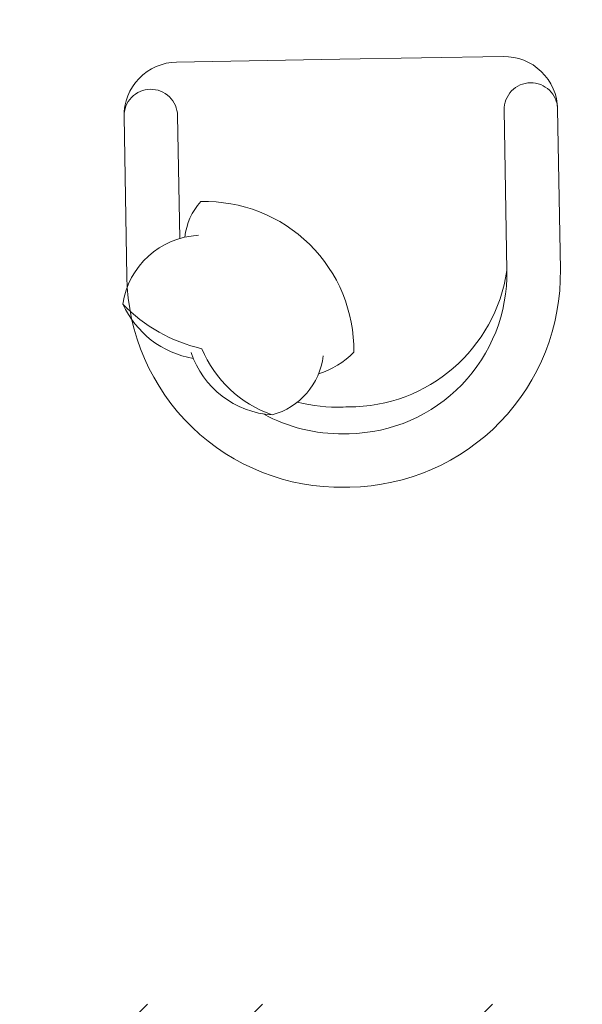
# Model space of a CAD drawing. Units: inches. Extents: x 963 to 2075, y 289 to 2657.
# Tile 49 of 98: x 1534 to 1556, y 1714 to 1752. Entities that reach past the tile are written whole.
import ezdxf

# ---------------------------------------------------------------- set-up
doc = ezdxf.new("R2010")
doc.units = ezdxf.units.IN
doc.layers.add('A-FURN', color=8, linetype='Continuous', lineweight=18)
doc.layers.add('A-WALL-PATT', color=8, linetype='Continuous', lineweight=13)

# ---------------------------------------------------------------- blocks, each defined once
blk = doc.blocks.new('ARMCHAIR-C')
at = {"ltscale": 0.03}
blk.add_lwpolyline([(8.609, -0.446), (2.235, -0.446, -0.414214), (0.146, 1.643), (0.146, 7.912, -0.414214), (8.504, 16.271), (8.609, 16.271), (8.713, 16.271, -0.414214), (17.072, 7.912), (17.072, 1.643, -0.414214), (14.982, -0.446), (8.609, -0.446)], format="xyb", dxfattribs=at)
for points in [[(2.235, 7.912, -0.414214), (8.504, 14.181), (8.609, 14.181)], [(11.825, 13.354, 0.130591), (8.713, 14.181), (8.609, 14.181)], [(2.235, 7.912, -0.372719), (8.504, 13.136), (8.609, 13.136)], [(10.495, 12.911, 0.072384), (8.713, 13.136), (8.609, 13.136)], [(14.611, 10.906, 0.306663), (11.495, 13.396, 0.30633), (9.459, 11.122, -0.872847)], [(17.243, 8.967, 0.14773), (14.189, 10.763, 0.213343), (11.495, 13.396, 0.178662)], [(14.776, 6.397, -0.165541), (14.129, 5.017, -0.425989), (8.261, 11.002, -0.121523), (9.654, 11.827, 7.115464)], [(14.249, 6.333, 0.356772), (17.243, 8.967, 0.249542), (14.53, 11.137, -9.61688)], [(2.235, 7.912), (2.235, 1.643, -0.414214), (1.191, 0.598), (1.191, 0.598, -0.414214), (0.146, 1.643)], [(14.982, 6.447), (14.982, 1.643, 0.414214), (16.027, 0.598), (16.027, 0.598, 0.414214), (17.072, 1.643)]]:
    blk.add_lwpolyline(points, format="xyb")

msp = doc.modelspace()

# ---------------------------------------------------------------- hatches: boundary and pattern name
at = {"layer": 'A-WALL-PATT'}
h = msp.add_hatch(dxfattribs=at)
h.set_pattern_fill('ANSI32', color=256)
h.paths.add_polyline_path([(1296.922, 2558.318), (1203.922, 2558.318), (1203.922, 2493.818), (1191.533, 2493.818), (1191.533, 2489.318), (1211.063, 2489.318), (1211.063, 2492.02), (1211.063, 2493.818), (1208.422, 2493.818), (1208.422, 2553.818), (1292.422, 2553.818), (1292.422, 2538.863), (1296.922, 2538.863)])
h.paths.add_polyline_path([(1442.422, 2558.318), (1349.422, 2558.318), (1349.422, 2538.943), (1353.922, 2538.943), (1353.922, 2553.818), (1437.922, 2553.818), (1437.922, 2493.818), (1434.542, 2493.818), (1434.542, 2489.318), (1448.311, 2489.318), (1448.311, 2491.568), (1448.311, 2493.818), (1442.422, 2493.818)])
h.paths.add_polyline_path([(1415.554, 2491.568), (1415.554, 2493.818), (1340.941, 2493.818), (1340.941, 2489.318), (1371.922, 2489.318), (1371.922, 2378.318), (1367.596, 2378.318), (1367.596, 2373.818), (1371.922, 2373.818), (1371.922, 2355.185), (1376.422, 2355.185), (1376.422, 2489.318), (1415.554, 2489.318)])
h.paths.add_polyline_path([(1304.941, 2491.568), (1304.941, 2493.818), (1296.922, 2493.818), (1296.922, 2514.863), (1292.422, 2514.863), (1292.422, 2493.818), (1232.808, 2493.818), (1232.808, 2489.318), (1256.422, 2489.318), (1256.422, 2327.318), (1253.714, 2327.318), (1253.714, 2322.818), (1328.422, 2322.818), (1328.422, 2331.147), (1323.922, 2331.147), (1323.922, 2327.318), (1260.922, 2327.318), (1260.922, 2373.818), (1323.922, 2373.818), (1323.922, 2357.812), (1328.422, 2357.812), (1328.422, 2373.818), (1346.007, 2373.818), (1346.007, 2376.068), (1346.007, 2378.318), (1260.922, 2378.318), (1260.922, 2489.318), (1304.941, 2489.318)])
h.paths.add_polyline_path([(1226.654, 2327.318), (1124.422, 2327.318), (1124.422, 2347.447), (1119.922, 2347.447), (1119.922, 2322.818), (1163.422, 2322.818), (1163.422, 2305.435), (1165.672, 2305.435), (1167.922, 2305.435), (1167.922, 2322.818), (1226.654, 2322.818), (1226.654, 2325.068)])
h.paths.add_polyline_path([(1095.922, 2489.318), (1124.422, 2489.318), (1131.533, 2489.318), (1131.533, 2491.568), (1131.533, 2493.818), (1119.922, 2493.818), (1091.422, 2493.818), (1091.422, 2417.318), (1095.922, 2417.318), (1119.922, 2417.318), (1119.922, 2407.447), (1124.422, 2407.447), (1124.422, 2421.818), (1095.922, 2421.818)])
h.paths.add_polyline_path([(1512.922, 2558.318), (1508.422, 2558.318), (1508.422, 2493.818), (1503.401, 2493.818), (1503.401, 2489.318), (1508.422, 2489.318), (1508.422, 2327.318), (1376.422, 2327.318), (1376.422, 2330.273), (1371.922, 2330.273), (1371.922, 2298.744), (1376.422, 2298.744), (1376.422, 2322.818), (1508.422, 2322.818), (1508.422, 2165.318), (1504.255, 2165.318), (1504.255, 2160.818), (1508.422, 2160.818), (1508.422, 2108.318), (1512.922, 2108.318), (1512.922, 2160.818), (1516.182, 2160.818), (1516.182, 2163.068), (1516.182, 2165.318), (1512.922, 2165.318), (1512.922, 2322.818), (1644.922, 2322.818), (1644.922, 2298.744), (1649.422, 2298.744), (1649.422, 2322.818), (1649.422, 2330.944), (1647.172, 2330.944), (1644.922, 2330.944), (1644.922, 2327.318), (1512.922, 2327.318), (1512.922, 2489.318), (1516.759, 2489.318), (1516.759, 2491.568), (1516.759, 2493.818), (1512.922, 2493.818)])
h.paths.add_polyline_path([(1671.922, 2558.318), (1578.922, 2558.318), (1578.922, 2493.818), (1573.526, 2493.818), (1573.526, 2489.318), (1586.537, 2489.318), (1586.537, 2491.568), (1586.537, 2493.818), (1583.422, 2493.818), (1583.422, 2553.818), (1667.422, 2553.818), (1667.422, 2541.109), (1671.922, 2541.109)])
h.paths.add_polyline_path([(1681.257, 2493.818), (1671.922, 2493.818), (1671.922, 2517.109), (1667.422, 2517.109), (1667.422, 2493.818), (1610.218, 2493.818), (1610.218, 2489.318), (1644.922, 2489.318), (1644.922, 2357.865), (1649.422, 2357.865), (1649.422, 2373.818), (1652.203, 2373.818), (1652.203, 2375.827), (1652.203, 2378.318), (1649.422, 2378.318), (1649.422, 2489.318), (1681.257, 2489.318), (1681.257, 2491.568)])
h.paths.add_polyline_path([(1821.922, 2558.318), (1728.922, 2558.318), (1728.922, 2541), (1733.422, 2541), (1733.422, 2553.818), (1817.422, 2553.818), (1817.422, 2493.818), (1813.507, 2493.818), (1813.507, 2489.318), (1830.078, 2489.318), (1830.078, 2491.568), (1830.078, 2493.818), (1821.922, 2493.818)])
h.paths.add_polyline_path([(1794.244, 2493.818), (1717.257, 2493.818), (1717.257, 2489.318), (1760.422, 2489.318), (1760.422, 2378.318), (1674.401, 2378.318), (1674.401, 2373.818), (1692.922, 2373.818), (1692.922, 2356.954), (1697.422, 2356.954), (1697.422, 2373.818), (1760.422, 2373.818), (1760.422, 2327.318), (1697.422, 2327.318), (1697.422, 2333.341), (1692.922, 2333.341), (1692.922, 2322.818), (1768.037, 2322.818), (1768.037, 2325.068), (1768.037, 2327.318), (1764.922, 2327.318), (1764.922, 2489.318), (1794.244, 2489.318)])
h.paths.add_polyline_path([(1733.422, 2517), (1728.922, 2517), (1728.922, 2493.818), (1733.422, 2493.818)], flags=17)
h.paths.add_polyline_path([(1929.922, 2493.818), (1890.078, 2493.818), (1890.078, 2489.318), (1896.922, 2489.318), (1925.422, 2489.318), (1925.422, 2421.818), (1896.922, 2421.818), (1896.922, 2408.318), (1901.422, 2408.318), (1901.422, 2417.318), (1925.422, 2417.318), (1929.922, 2417.318)])
h.paths.add_polyline_path([(1901.422, 2348.318), (1896.922, 2348.318), (1896.922, 2327.318), (1800.423, 2327.318), (1800.423, 2322.818), (1853.422, 2322.818), (1853.422, 2309.453), (1857.922, 2309.453), (1857.922, 2322.818), (1901.422, 2322.818)])
h.paths.add_polyline_path([(1857.922, 2249.453), (1853.422, 2249.453), (1853.422, 2214.818), (1686.309, 2214.818), (1686.309, 2210.318), (1853.422, 2210.318), (1853.422, 2202.134), (1857.922, 2202.134), (1857.922, 2210.318)])
h.paths.add_polyline_path([(1857.922, 2142.134), (1853.422, 2142.134), (1853.422, 2115.422), (1841.422, 2115.422), (1841.422, 2088.531), (1841.422, 2046.949), (1845.922, 2046.949), (1845.922, 2110.922), (1905.922, 2110.922), (1905.922, 2092.517), (1910.422, 2092.517), (1910.422, 2115.422), (1857.922, 2115.422)])
h.paths.add_polyline_path([(1532.436, 1482.342), (1573.456, 1482.342), (1573.456, 1501), (1532.436, 1501)], flags=9)
h.paths.add_polyline_path([(1438.658, 1486.302), (1479.678, 1486.302), (1479.678, 1504.96), (1438.658, 1504.96)], flags=9)
h.paths.add_polyline_path([(1411.215, 1365.308), (1659.139, 1365.308), (1659.139, 1402.401), (1411.215, 1402.401)], flags=9)
h.paths.add_polyline_path([(1185.671, 2296.298), (1248.16, 2296.298), (1248.16, 2314.955), (1185.671, 2314.955)], flags=9)
h.paths.add_polyline_path([(1177.31, 2187.35), (1216.15, 2187.35), (1216.15, 2206.007), (1177.31, 2206.007)], flags=9)
h.paths.add_polyline_path([(1295.101, 1602.083), (1328.26, 1602.083), (1328.26, 1620.741), (1295.101, 1620.741)], flags=9)
h.paths.add_polyline_path([(1525.126, 2005.99), (1558.39, 2005.99), (1558.39, 2024.648), (1525.126, 2024.648)], flags=9)
h.paths.add_polyline_path([(1459.606, 1977.125), (1472.195, 1977.125), (1472.195, 1987.429), (1459.606, 1987.429)], flags=9)
h.paths.add_polyline_path([(1467.815, 2053.676), (1480.018, 2053.676), (1480.018, 2063.979), (1467.815, 2063.979)], flags=9)
h.paths.add_polyline_path([(1555.184, 2119.02), (1584.563, 2119.02), (1584.563, 2137.678), (1555.184, 2137.678)], flags=25)
h.paths.add_polyline_path([(1405.389, 2115.291), (1444.478, 2115.291), (1444.478, 2133.948), (1405.389, 2133.948)], flags=25)
h.paths.add_polyline_path([(1698.482, 2004.259), (1727.695, 2004.259), (1727.695, 2022.916), (1698.482, 2022.916)], flags=9)
h.paths.add_polyline_path([(1612.158, 1972.855), (1629.016, 1972.855), (1629.016, 1983.159), (1612.158, 1983.159)], flags=9)
h.paths.add_polyline_path([(1608.289, 2060.036), (1625.147, 2060.036), (1625.147, 2070.34), (1608.289, 2070.34)], flags=9)
h.paths.add_polyline_path([(1527.954, 1684.402), (1566.795, 1684.402), (1566.795, 1703.06), (1527.954, 1703.06)], flags=9)
h.paths.add_polyline_path([(1422.792, 1683.59), (1461.633, 1683.59), (1461.633, 1702.247), (1422.792, 1702.247)], flags=9)
h.paths.add_polyline_path([(1531.262, 1732.459), (1574.015, 1732.459), (1574.015, 1751.116), (1531.262, 1751.116)], flags=9)
h.paths.add_polyline_path([(1402.872, 1732.845), (1439.799, 1732.845), (1439.799, 1751.502), (1402.872, 1751.502)], flags=9)
h.paths.add_polyline_path([(1243.122, 1923.132), (1281.962, 1923.132), (1281.962, 1941.79), (1243.122, 1941.79)], flags=9)
h.paths.add_polyline_path([(1181.752, 1792.268), (1244.241, 1792.268), (1244.241, 1810.926), (1181.752, 1810.926)], flags=9)
h.paths.add_polyline_path([(1265.822, 1670.3), (1316.071, 1670.3), (1316.071, 1688.957), (1265.822, 1688.957)], flags=9)
h.paths.add_polyline_path([(1140.263, 1676.054), (1179.104, 1676.054), (1179.104, 1694.711), (1140.263, 1694.711)], flags=9)
h.paths.add_polyline_path([(1107.49, 1490.889), (1143.374, 1490.889), (1143.374, 1509.546), (1107.49, 1509.546)], flags=9)
h.paths.add_polyline_path([(1217.584, 1483.899), (1246.741, 1483.899), (1246.741, 1502.556), (1217.584, 1502.556)], flags=9)
h.paths.add_polyline_path([(1389.21, 1486.919), (1418.367, 1486.919), (1418.367, 1505.576), (1389.21, 1505.576)], flags=9)
h.paths.add_polyline_path([(1672.208, 1602.083), (1705.366, 1602.083), (1705.366, 1620.741), (1672.208, 1620.741)], flags=9)
h.paths.add_polyline_path([(1752.082, 1522.638), (1781.24, 1522.638), (1781.24, 1541.295), (1752.082, 1541.295)], flags=9)
h.paths.add_polyline_path([(1848.275, 1491.26), (1884.158, 1491.26), (1884.158, 1509.918), (1848.275, 1509.918)], flags=9)
h.paths.add_polyline_path([(1822.47, 1685.62), (1861.31, 1685.62), (1861.31, 1704.278), (1822.47, 1704.278)], flags=9)
h.paths.add_polyline_path([(1713.195, 1672.232), (1763.444, 1672.232), (1763.444, 1690.889), (1713.195, 1690.889)], flags=9)
h.paths.add_polyline_path([(1736.619, 1790.578), (1799.109, 1790.578), (1799.109, 1809.235), (1736.619, 1809.235)], flags=9)
h.paths.add_polyline_path([(1691.491, 1916.355), (1730.332, 1916.355), (1730.332, 1935.013), (1691.491, 1935.013)], flags=9)
h.paths.add_polyline_path([(1764.872, 1973.922), (1794.306, 1973.922), (1794.306, 1992.58), (1764.872, 1992.58)], flags=9)
h.paths.add_polyline_path([(1767.854, 2034.017), (1797.288, 2034.017), (1797.288, 2052.674), (1767.854, 2052.674)], flags=9)
h.paths.add_polyline_path([(1851.593, 2060.331), (1880.751, 2060.331), (1880.751, 2078.989), (1851.593, 2078.989)], flags=25)
h.paths.add_polyline_path([(1688.491, 2086.874), (1727.332, 2086.874), (1727.332, 2105.531), (1688.491, 2105.531)], flags=9)
h.paths.add_polyline_path([(1537.743, 2293.581), (1580.495, 2293.581), (1580.495, 2312.239), (1537.743, 2312.239)], flags=25)
h.paths.add_polyline_path([(1425.587, 2296.109), (1468.34, 2296.109), (1468.34, 2314.766), (1425.587, 2314.766)], flags=25)
h.paths.add_polyline_path([(1278.518, 2004.184), (1307.72, 2004.184), (1307.72, 2022.841), (1278.518, 2022.841)], flags=9)
h.paths.add_polyline_path([(1193.282, 1973.635), (1222.715, 1973.635), (1222.715, 1992.292), (1193.282, 1992.292)], flags=9)
h.paths.add_polyline_path([(1192.411, 2040.577), (1221.845, 2040.577), (1221.845, 2059.234), (1192.411, 2059.234)], flags=9)
h.paths.add_polyline_path([(1130.603, 1951.393), (1159.76, 1951.393), (1159.76, 1970.05), (1130.603, 1970.05)], flags=9)
h.paths.add_polyline_path([(1132.827, 2052.494), (1161.984, 2052.494), (1161.984, 2071.151), (1132.827, 2071.151)], flags=9)
h.paths.add_polyline_path([(1265.128, 2334.619), (1315.377, 2334.619), (1315.377, 2353.277), (1265.128, 2353.277)], flags=25)
h.paths.add_polyline_path([(1136.741, 2330.785), (1175.582, 2330.785), (1175.582, 2349.443), (1136.741, 2349.443)], flags=9)
h.paths.add_polyline_path([(1287.422, 2417.204), (1320.58, 2417.204), (1320.58, 2435.861), (1287.422, 2435.861)], flags=25)
h.paths.add_polyline_path([(1430.988, 2329.159), (1469.828, 2329.159), (1469.828, 2347.816), (1430.988, 2347.816)], flags=25)
h.paths.add_polyline_path([(1525.424, 2329.213), (1564.264, 2329.213), (1564.264, 2347.87), (1525.424, 2347.87)], flags=25)
h.paths.add_polyline_path([(1684.525, 2382.799), (1717.683, 2382.799), (1717.683, 2401.457), (1684.525, 2401.457)], flags=25)
h.paths.add_polyline_path([(1704.805, 2340.293), (1755.054, 2340.293), (1755.054, 2358.95), (1704.805, 2358.95)], flags=25)
h.paths.add_polyline_path([(1694.113, 2287.757), (1756.602, 2287.757), (1756.602, 2306.414), (1694.113, 2306.414)], flags=9)
h.paths.add_polyline_path([(1815.778, 2329.861), (1854.618, 2329.861), (1854.618, 2348.518), (1815.778, 2348.518)], flags=9)
h.paths.add_polyline_path([(1842.873, 2514.256), (1878.756, 2514.256), (1878.756, 2532.914), (1842.873, 2532.914)], flags=9)
h.paths.add_polyline_path([(1769.513, 2531.447), (1798.671, 2531.447), (1798.671, 2550.104), (1769.513, 2550.104)], flags=25)
h.paths.add_polyline_path([(1594.772, 2518.468), (1623.93, 2518.468), (1623.93, 2537.125), (1594.772, 2537.125)], flags=25)
h.paths.add_polyline_path([(1520.723, 2516.185), (1556.606, 2516.185), (1556.606, 2534.842), (1520.723, 2534.842)], flags=25)
h.paths.add_polyline_path([(1464.456, 2516.694), (1500.34, 2516.694), (1500.34, 2535.351), (1464.456, 2535.351)], flags=25)
h.paths.add_polyline_path([(1365.696, 2528.97), (1394.854, 2528.97), (1394.854, 2547.627), (1365.696, 2547.627)], flags=25)
h.paths.add_polyline_path([(1222.838, 2516.231), (1251.995, 2516.231), (1251.995, 2534.889), (1222.838, 2534.889)], flags=25)
h.paths.add_polyline_path([(1104.545, 2509.6), (1140.429, 2509.6), (1140.429, 2528.257), (1104.545, 2528.257)], flags=9)
h = msp.add_hatch(dxfattribs=at)
h.set_pattern_fill('ANSI32', color=256)
h.paths.add_polyline_path([(1335.968, 2212.568), (1335.968, 2214.818), (1167.922, 2214.818), (1167.922, 2245.435), (1163.422, 2245.435), (1163.422, 2210.318), (1163.422, 2194.812), (1167.922, 2194.812), (1167.922, 2210.318), (1335.968, 2210.318)])
h.paths.add_polyline_path([(1532.436, 1482.342), (1573.456, 1482.342), (1573.456, 1501), (1532.436, 1501)], flags=9)
h.paths.add_polyline_path([(1438.658, 1486.302), (1479.678, 1486.302), (1479.678, 1504.96), (1438.658, 1504.96)], flags=9)
h.paths.add_polyline_path([(1411.215, 1365.308), (1659.139, 1365.308), (1659.139, 1402.401), (1411.215, 1402.401)], flags=9)
h.paths.add_polyline_path([(1185.671, 2296.298), (1248.16, 2296.298), (1248.16, 2314.955), (1185.671, 2314.955)], flags=9)
h.paths.add_polyline_path([(1177.31, 2187.35), (1216.15, 2187.35), (1216.15, 2206.007), (1177.31, 2206.007)], flags=9)
h.paths.add_polyline_path([(1295.101, 1602.083), (1328.26, 1602.083), (1328.26, 1620.741), (1295.101, 1620.741)], flags=9)
h.paths.add_polyline_path([(1525.126, 2005.99), (1558.39, 2005.99), (1558.39, 2024.648), (1525.126, 2024.648)], flags=9)
h.paths.add_polyline_path([(1459.606, 1977.125), (1472.195, 1977.125), (1472.195, 1987.429), (1459.606, 1987.429)], flags=9)
h.paths.add_polyline_path([(1467.815, 2053.676), (1480.018, 2053.676), (1480.018, 2063.979), (1467.815, 2063.979)], flags=9)
h.paths.add_polyline_path([(1555.184, 2119.02), (1584.563, 2119.02), (1584.563, 2137.678), (1555.184, 2137.678)], flags=9)
h.paths.add_polyline_path([(1405.389, 2115.291), (1444.478, 2115.291), (1444.478, 2133.948), (1405.389, 2133.948)], flags=9)
h.paths.add_polyline_path([(1698.482, 2004.259), (1727.695, 2004.259), (1727.695, 2022.916), (1698.482, 2022.916)], flags=9)
h.paths.add_polyline_path([(1612.158, 1972.855), (1629.016, 1972.855), (1629.016, 1983.159), (1612.158, 1983.159)], flags=9)
h.paths.add_polyline_path([(1608.289, 2060.036), (1625.147, 2060.036), (1625.147, 2070.34), (1608.289, 2070.34)], flags=9)
h.paths.add_polyline_path([(1527.954, 1684.402), (1566.795, 1684.402), (1566.795, 1703.06), (1527.954, 1703.06)], flags=9)
h.paths.add_polyline_path([(1422.792, 1683.59), (1461.633, 1683.59), (1461.633, 1702.247), (1422.792, 1702.247)], flags=9)
h.paths.add_polyline_path([(1531.262, 1732.459), (1574.015, 1732.459), (1574.015, 1751.116), (1531.262, 1751.116)], flags=9)
h.paths.add_polyline_path([(1402.872, 1732.845), (1439.799, 1732.845), (1439.799, 1751.502), (1402.872, 1751.502)], flags=9)
h.paths.add_polyline_path([(1243.122, 1923.132), (1281.962, 1923.132), (1281.962, 1941.79), (1243.122, 1941.79)], flags=9)
h.paths.add_polyline_path([(1181.752, 1792.268), (1244.241, 1792.268), (1244.241, 1810.926), (1181.752, 1810.926)], flags=9)
h.paths.add_polyline_path([(1265.822, 1670.3), (1316.071, 1670.3), (1316.071, 1688.957), (1265.822, 1688.957)], flags=9)
h.paths.add_polyline_path([(1140.263, 1676.054), (1179.104, 1676.054), (1179.104, 1694.711), (1140.263, 1694.711)], flags=9)
h.paths.add_polyline_path([(1107.49, 1490.889), (1143.374, 1490.889), (1143.374, 1509.546), (1107.49, 1509.546)], flags=9)
h.paths.add_polyline_path([(1217.584, 1483.899), (1246.741, 1483.899), (1246.741, 1502.556), (1217.584, 1502.556)], flags=9)
h.paths.add_polyline_path([(1389.21, 1486.919), (1418.367, 1486.919), (1418.367, 1505.576), (1389.21, 1505.576)], flags=9)
h.paths.add_polyline_path([(1672.208, 1602.083), (1705.366, 1602.083), (1705.366, 1620.741), (1672.208, 1620.741)], flags=9)
h.paths.add_polyline_path([(1752.082, 1522.638), (1781.24, 1522.638), (1781.24, 1541.295), (1752.082, 1541.295)], flags=9)
h.paths.add_polyline_path([(1848.275, 1491.26), (1884.158, 1491.26), (1884.158, 1509.918), (1848.275, 1509.918)], flags=9)
h.paths.add_polyline_path([(1822.47, 1685.62), (1861.31, 1685.62), (1861.31, 1704.278), (1822.47, 1704.278)], flags=9)
h.paths.add_polyline_path([(1713.195, 1672.232), (1763.444, 1672.232), (1763.444, 1690.889), (1713.195, 1690.889)], flags=9)
h.paths.add_polyline_path([(1736.619, 1790.578), (1799.109, 1790.578), (1799.109, 1809.235), (1736.619, 1809.235)], flags=9)
h.paths.add_polyline_path([(1691.491, 1916.355), (1730.332, 1916.355), (1730.332, 1935.013), (1691.491, 1935.013)], flags=9)
h.paths.add_polyline_path([(1764.872, 1973.922), (1794.306, 1973.922), (1794.306, 1992.58), (1764.872, 1992.58)], flags=9)
h.paths.add_polyline_path([(1767.854, 2034.017), (1797.288, 2034.017), (1797.288, 2052.674), (1767.854, 2052.674)], flags=9)
h.paths.add_polyline_path([(1851.593, 2060.331), (1880.751, 2060.331), (1880.751, 2078.989), (1851.593, 2078.989)], flags=9)
h.paths.add_polyline_path([(1688.491, 2086.874), (1727.332, 2086.874), (1727.332, 2105.531), (1688.491, 2105.531)], flags=9)
h.paths.add_polyline_path([(1537.743, 2293.581), (1580.495, 2293.581), (1580.495, 2312.239), (1537.743, 2312.239)], flags=9)
h.paths.add_polyline_path([(1425.587, 2296.109), (1468.34, 2296.109), (1468.34, 2314.766), (1425.587, 2314.766)], flags=9)
h.paths.add_polyline_path([(1278.518, 2004.184), (1307.72, 2004.184), (1307.72, 2022.841), (1278.518, 2022.841)], flags=9)
h.paths.add_polyline_path([(1193.282, 1973.635), (1222.715, 1973.635), (1222.715, 1992.292), (1193.282, 1992.292)], flags=9)
h.paths.add_polyline_path([(1192.411, 2040.577), (1221.845, 2040.577), (1221.845, 2059.234), (1192.411, 2059.234)], flags=9)
h.paths.add_polyline_path([(1130.603, 1951.393), (1159.76, 1951.393), (1159.76, 1970.05), (1130.603, 1970.05)], flags=9)
h.paths.add_polyline_path([(1132.827, 2052.494), (1161.984, 2052.494), (1161.984, 2071.151), (1132.827, 2071.151)], flags=9)
h.paths.add_polyline_path([(1265.128, 2334.619), (1315.377, 2334.619), (1315.377, 2353.277), (1265.128, 2353.277)], flags=9)
h.paths.add_polyline_path([(1136.741, 2330.785), (1175.582, 2330.785), (1175.582, 2349.443), (1136.741, 2349.443)], flags=9)
h.paths.add_polyline_path([(1287.422, 2417.204), (1320.58, 2417.204), (1320.58, 2435.861), (1287.422, 2435.861)], flags=9)
h.paths.add_polyline_path([(1430.988, 2329.159), (1469.828, 2329.159), (1469.828, 2347.816), (1430.988, 2347.816)], flags=9)
h.paths.add_polyline_path([(1525.424, 2329.213), (1564.264, 2329.213), (1564.264, 2347.87), (1525.424, 2347.87)], flags=9)
h.paths.add_polyline_path([(1684.525, 2382.799), (1717.683, 2382.799), (1717.683, 2401.457), (1684.525, 2401.457)], flags=9)
h.paths.add_polyline_path([(1704.805, 2340.293), (1755.054, 2340.293), (1755.054, 2358.95), (1704.805, 2358.95)], flags=9)
h.paths.add_polyline_path([(1694.113, 2287.757), (1756.602, 2287.757), (1756.602, 2306.414), (1694.113, 2306.414)], flags=9)
h.paths.add_polyline_path([(1815.778, 2329.861), (1854.618, 2329.861), (1854.618, 2348.518), (1815.778, 2348.518)], flags=9)
h.paths.add_polyline_path([(1842.873, 2514.256), (1878.756, 2514.256), (1878.756, 2532.914), (1842.873, 2532.914)], flags=9)
h.paths.add_polyline_path([(1769.513, 2531.447), (1798.671, 2531.447), (1798.671, 2550.104), (1769.513, 2550.104)], flags=9)
h.paths.add_polyline_path([(1594.772, 2518.468), (1623.93, 2518.468), (1623.93, 2537.125), (1594.772, 2537.125)], flags=9)
h.paths.add_polyline_path([(1520.723, 2516.185), (1556.606, 2516.185), (1556.606, 2534.842), (1520.723, 2534.842)], flags=9)
h.paths.add_polyline_path([(1464.456, 2516.694), (1500.34, 2516.694), (1500.34, 2535.351), (1464.456, 2535.351)], flags=9)
h.paths.add_polyline_path([(1365.696, 2528.97), (1394.854, 2528.97), (1394.854, 2547.627), (1365.696, 2547.627)], flags=9)
h.paths.add_polyline_path([(1222.838, 2516.231), (1251.995, 2516.231), (1251.995, 2534.889), (1222.838, 2534.889)], flags=9)
h.paths.add_polyline_path([(1104.545, 2509.6), (1140.429, 2509.6), (1140.429, 2528.257), (1104.545, 2528.257)], flags=9)
h = msp.add_hatch(dxfattribs=at)
h.set_pattern_fill('ANSI32', color=256)
h.paths.add_polyline_path([(1473.609, 2163.068), (1473.609, 2165.318), (1376.422, 2165.318), (1376.422, 2227.983), (1371.922, 2227.983), (1371.922, 2214.818), (1368.405, 2214.818), (1368.405, 2210.318), (1371.922, 2210.318), (1371.922, 2160.818), (1395.922, 2160.818), (1395.922, 2090.318), (1217.345, 2090.318), (1217.345, 2085.818), (1395.922, 2085.818), (1458.922, 2085.818), (1458.922, 2108.318), (1454.422, 2108.318), (1454.422, 2090.318), (1400.422, 2090.318), (1400.422, 2160.818), (1473.609, 2160.818)])
h.paths.add_polyline_path([(1649.422, 2210.318), (1653.225, 2210.318), (1653.225, 2214.818), (1649.422, 2214.818), (1649.422, 2227.983), (1644.922, 2227.983), (1644.922, 2165.318), (1550.099, 2165.318), (1550.099, 2160.818), (1620.922, 2160.818), (1620.922, 2112.818), (1555.446, 2112.818), (1555.446, 2108.318), (1584.327, 2108.318), (1584.327, 2084.916), (1588.827, 2084.916), (1588.827, 2108.318), (1625.422, 2108.318), (1667.951, 2108.318), (1667.951, 2022.667), (1588.827, 2022.667), (1588.827, 2047.408), (1584.327, 2047.408), (1584.327, 1996.003), (1588.827, 1996.003), (1588.827, 2018.318), (1667.951, 2018.167), (1667.951, 1928.318), (1625.422, 1928.318), (1625.422, 1923.818), (1672.451, 1923.818), (1672.451, 1928.318), (1672.451, 1946.663), (1785.446, 1946.663), (1785.446, 1951.163), (1743.034, 1951.163), (1743.034, 2017.922), (1841.422, 2017.922), (1841.422, 2014.775), (1845.922, 2014.775), (1845.922, 2017.922), (1905.922, 2017.922), (1905.922, 1987.511), (1910.422, 1987.511), (1910.422, 2022.422), (1910.422, 2068.517), (1905.922, 2068.517), (1905.922, 2022.422), (1845.922, 2022.422), (1845.922, 2025.851), (1843.672, 2025.851), (1841.422, 2025.851), (1841.422, 2022.422), (1743.034, 2022.422), (1743.034, 2084.031), (1768.451, 2084.031), (1785.446, 2084.031), (1785.446, 2088.531), (1672.451, 2088.531), (1672.451, 2112.818), (1667.951, 2112.818), (1625.422, 2112.818), (1625.422, 2160.818), (1649.422, 2160.818)])
h.paths.add_polyline_path([(1672.451, 2084.031), (1738.534, 2084.031), (1738.534, 1951.163), (1672.451, 1951.163)], flags=16)
h.paths.add_polyline_path([(1672.451, 2084.031), (1738.534, 2084.031), (1705.492, 2017.597)], flags=0)
h.paths.add_polyline_path([(1262.766, 2085.818), (1258.266, 2085.818), (1258.266, 2023.278), (1184.422, 2023.278), (1184.422, 2018.778), (1258.266, 2018.778), (1258.266, 1950.818), (1262.766, 1950.818)])
h.paths.add_polyline_path([(1312.266, 2085.818), (1307.766, 2085.818), (1307.766, 1950.818), (1312.266, 1950.818)])
h.paths.add_polyline_path([(1458.922, 1950.818), (1395.922, 1950.818), (1216.568, 1950.818), (1216.568, 1946.318), (1346.422, 1946.318), (1395.922, 1946.318), (1395.922, 1875.818), (1371.922, 1875.818), (1371.922, 1826.318), (1368.931, 1826.318), (1368.931, 1821.818), (1371.922, 1821.818), (1371.922, 1813.622), (1376.422, 1813.622), (1376.422, 1871.318), (1474.504, 1871.318), (1474.504, 1873.568), (1474.504, 1875.818), (1400.422, 1875.818), (1400.422, 1946.318), (1454.422, 1946.318), (1454.422, 1928.318), (1458.922, 1928.318)])
h.paths.add_polyline_path([(1184.422, 2120.778), (1167.922, 2120.778), (1167.922, 2134.812), (1165.672, 2134.812), (1163.422, 2134.812), (1163.422, 2120.778), (1119.922, 2120.778), (1119.922, 2098.095), (1124.422, 2098.095), (1124.422, 2116.278), (1167.922, 2116.278), (1179.922, 2116.278), (1179.922, 2045.916), (1184.422, 2045.916), (1184.422, 2090.318), (1184.422, 2116.278)])
h.paths.add_polyline_path([(1124.422, 2018.778), (1179.922, 2018.778), (1179.922, 2016.294), (1184.422, 2016.294), (1184.422, 2023.278), (1184.422, 2026.588), (1182.172, 2026.588), (1179.922, 2026.588), (1179.922, 2023.278), (1124.422, 2023.278), (1124.422, 2074.095), (1119.922, 2074.095), (1119.922, 2018.778), (1119.922, 1979.633), (1124.422, 1979.633)])
h.paths.add_polyline_path([(1184.422, 1925.778), (1184.422, 1946.318), (1184.422, 1996.073), (1182.172, 1996.073), (1179.922, 1996.073), (1179.922, 1925.778), (1124.422, 1925.778), (1124.422, 1955.633), (1119.922, 1955.502), (1119.922, 1921.278), (1158.922, 1921.278), (1158.922, 1909.983), (1163.422, 1909.983), (1163.422, 1921.278), (1184.422, 1921.278)])
h.paths.add_polyline_path([(1341.449, 1826.318), (1163.422, 1826.318), (1163.422, 1849.983), (1158.922, 1849.983), (1158.922, 1821.818), (1158.922, 1804.033), (1163.422, 1804.033), (1163.422, 1821.818), (1341.449, 1821.818)])
h.paths.add_polyline_path([(1222.981, 1713.818), (1163.422, 1713.818), (1163.422, 1744.033), (1161.172, 1744.033), (1158.922, 1744.033), (1158.922, 1713.818), (1119.922, 1713.818), (1119.922, 1694.65), (1124.422, 1694.65), (1124.422, 1709.318), (1158.922, 1709.318), (1222.981, 1709.318)])
h.paths.add_polyline_path([(1328.422, 1713.818), (1252.042, 1713.818), (1252.042, 1711.568), (1252.042, 1709.318), (1256.422, 1709.318), (1256.422, 1547.318), (1232.937, 1547.318), (1232.937, 1545.068), (1232.937, 1542.818), (1292.422, 1542.818), (1292.422, 1527.634), (1296.922, 1527.634), (1296.922, 1542.818), (1299.464, 1542.818), (1299.464, 1547.318), (1260.922, 1547.318), (1260.922, 1658.318), (1343.661, 1658.318), (1343.661, 1660.568), (1343.661, 1662.818), (1328.422, 1662.818), (1328.422, 1676.589), (1327.402, 1676.589), (1323.922, 1676.589), (1323.922, 1662.818), (1260.922, 1662.818), (1260.922, 1709.318), (1323.922, 1709.318), (1323.922, 1699.851), (1328.422, 1699.851)])
h.paths.add_polyline_path([(1649.422, 1875.818), (1625.422, 1875.818), (1625.422, 1928.318), (1620.922, 1928.318), (1588.827, 1928.318), (1588.827, 1950.59), (1584.327, 1950.59), (1584.327, 1928.318), (1555.446, 1928.318), (1555.446, 1923.818), (1620.922, 1923.818), (1620.922, 1875.818), (1548.952, 1875.818), (1548.952, 1873.568), (1548.952, 1871.318), (1644.922, 1871.318), (1644.922, 1813.622), (1649.422, 1813.622), (1649.422, 1821.818), (1652.045, 1821.818), (1652.045, 1824.068), (1652.045, 1826.318), (1649.422, 1826.318)])
h.paths.add_polyline_path([(1512.922, 1871.318), (1516.476, 1871.318), (1516.476, 1875.818), (1512.922, 1875.818), (1512.922, 1923.818), (1512.922, 1928.318), (1512.922, 1930.827), (1508.422, 1930.827), (1508.422, 1875.818), (1504.411, 1875.818), (1504.411, 1871.318), (1508.422, 1871.318), (1508.422, 1713.818), (1376.422, 1713.818), (1376.422, 1743.325), (1371.922, 1743.325), (1371.922, 1709.318), (1371.922, 1706.01), (1376.422, 1706.01), (1376.422, 1709.318), (1508.422, 1709.318), (1508.422, 1547.318), (1501.871, 1547.318), (1501.871, 1542.818), (1508.422, 1542.818), (1508.422, 1482.818), (1508.422, 1436.318), (1512.922, 1436.318), (1512.922, 1542.818), (1519.318, 1542.818), (1519.318, 1545.068), (1519.318, 1547.318), (1512.922, 1547.318), (1512.922, 1709.318), (1644.922, 1709.318), (1644.922, 1707.548), (1649.422, 1707.548), (1649.422, 1709.318), (1649.422, 1743.325), (1644.922, 1743.325), (1644.922, 1713.818), (1512.922, 1713.818)])
h.paths.add_polyline_path([(1129.884, 1545.068), (1129.884, 1547.318), (1124.422, 1547.318), (1095.922, 1547.318), (1095.922, 1614.818), (1124.422, 1614.818), (1124.422, 1619.318), (1095.922, 1619.318), (1091.422, 1619.318), (1091.422, 1542.818), (1095.922, 1542.818), (1119.922, 1542.818), (1129.884, 1542.818)])
h.paths.add_polyline_path([(1208.422, 1542.818), (1211.74, 1542.818), (1211.74, 1547.318), (1198.851, 1547.318), (1198.851, 1542.818), (1203.922, 1542.818), (1203.922, 1478.318), (1208.422, 1478.318), (1296.922, 1478.318), (1296.922, 1503.634), (1292.422, 1503.634), (1292.422, 1482.818), (1208.422, 1482.818)])
h.paths.add_polyline_path([(1430.422, 1542.818), (1435.699, 1542.818), (1435.699, 1545.068), (1435.699, 1547.318), (1422.658, 1547.318), (1422.658, 1545.068), (1422.658, 1542.818), (1425.922, 1542.818), (1425.922, 1482.857), (1341.922, 1482.857), (1341.922, 1502.732), (1337.422, 1502.732), (1337.422, 1478.357), (1425.922, 1478.357), (1425.922, 1440.818), (1425.922, 1436.318), (1430.422, 1436.318)])
h.paths.add_polyline_path([(1698.482, 2004.259), (1727.695, 2004.259), (1727.695, 2022.916), (1698.482, 2022.916)], flags=8)

# ---------------------------------------------------------------- block references
at = {"layer": 'A-FURN', "rotation": 180.9834642143791}
msp.add_blockref('ARMCHAIR-C', (1554.83, 1750.432), dxfattribs=at)

doc.saveas('drawing.dxf')
